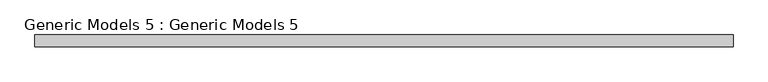
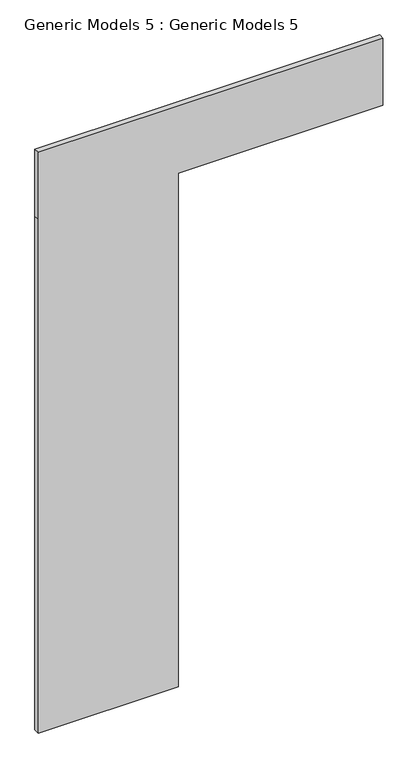
"""IFC4 building model written with IfcOpenShell, lengths in millimetres: proxy geometry, Generic Models 5 : Generic Models 5."""

from ifc_helpers import new_model, si_unit, frame, origin, place, context, project, spatial, polyline, outline, extrude, source, transform, mapped, element, save


def generic_models_5_generic_models_5_f46b040b(model_context):
    return source(origin(), model_context, "Body", "SweptSolid", [
        extrude(outline(polyline([(7924.8, -3859.560819), (7010.4, -3859.560819), (0.0, -3859.560819), (0.0, -2052.0455733), (7010.4, -2052.0455733), (7010.4, 589.554407), (7924.8, 589.554407), (7924.8, -3859.560819)])), frame((0.0, -4187.674389, 0.0), z_axis=(0.0, 1.0, 0.0), x_axis=(0.0, 0.0, 1.0)), (0.0, 0.0, 1.0), 76.2),
    ])


if __name__ == "__main__":
    model = new_model("IFC4")
    model_context = context("Model", 3, world=origin())
    ifc_project = project(units=[si_unit("LENGTHUNIT", "METRE", prefix="MILLI")], contexts=[model_context])
    site = spatial("IfcSite", under=ifc_project)
    building = spatial("IfcBuilding", under=site)
    placement = place(None, origin())
    generic_models_5_generic_models_5_shape = generic_models_5_generic_models_5_f46b040b(model_context)
    element("IfcBuildingElementProxy", 1, Name="Generic Models 5 : Generic Models 5", ObjectType="Generic Models 5 : Generic Models 5", at=placement, inside=building, context=model_context, shape_type="MappedRepresentation", body=[
        mapped(generic_models_5_generic_models_5_shape, transform((0.0, 0.0, 0.0), x_axis=(1.0, 0.0, 0.0), y_axis=(0.0, 1.0, 0.0), z_axis=(0.0, 0.0, 1.0))),
    ])
    save(model, "model.ifc")
